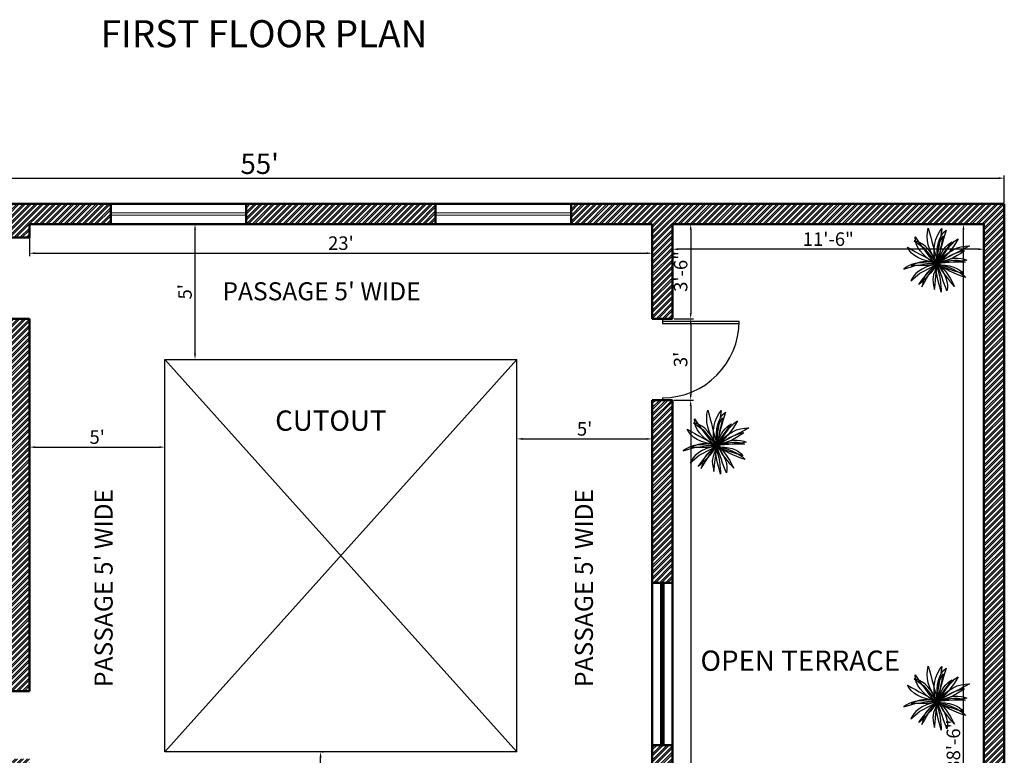
# Model space of a CAD drawing. Units: inches. Extents: x 3590 to 5167, y 65 to 1917.
# Tile 25 of 100: x 4644 to 5080, y 971 to 1297. Entities that reach past the tile are written whole.
import ezdxf

# ---------------------------------------------------------------- set-up
doc = ezdxf.new("R2010")
doc.units = ezdxf.units.IN
for name, color, linetype, lineweight in [('A-ANNO-DIMS', 2, 'Continuous', 18), ('A-ANNO-TEXT', 7, 'Continuous', 25), ('A-AREA-IDEN', 7, 'Continuous', 18), ('A-DOOR', 3, 'Continuous', 25), ('A-FLOR-OTLN', 7, 'Continuous', 25), ('A-GLAZ', 4, 'Continuous', 18), ('A-WALL', 7, 'Continuous', 50), ('A-WALL-PATT', 251, 'Continuous', 13), ('L-PLNT', 94, 'Continuous', 18)]:
    doc.layers.add(name, color=color, linetype=linetype, lineweight=lineweight)
doc.layers.add('DIENHOA', color=3, linetype='Continuous')
doc.styles.get("Standard").update_dxf_attribs({"font": 'arial.ttf'})
doc.dimstyles.new('ISO-25', dxfattribs={"dimtxt": 9, "dimasz": 2.5, "dimexe": 1.25, "dimexo": 0.625, "dimtad": 1, "dimdec": 1, "dimlunit": 3, "dimtxsty": 'Standard', "dimcen": 2.5, "dimadec": 0, "dimazin": 0, "dimtfac": 1, "dimtdec": 1, "dimtmove": 0, "dimatfit": 3, "dimfxl": 1, "dimarcsym": 0})

# ---------------------------------------------------------------- blocks, each defined once
blk = doc.blocks.new('*D105')
at = {"layer": 'A-ANNO-DIMS', "color": 0, "lineweight": -2, "transparency": 16777216}
for p, q in [((4420.27, 1215.97), (4420.27, 1227.96)), ((4422.77, 1226.71), (5077.77, 1226.71)), ((5080.27, 1215.97), (5080.27, 1227.96))]:
    blk.add_line(p, q, dxfattribs=at)
at = {"layer": 'A-ANNO-DIMS', "color": 0, "transparency": 16777216}
for points in [[(4422.77, 1227.13), (4422.77, 1226.29), (4420.27, 1226.71)], [(5077.77, 1227.13), (5077.77, 1226.29), (5080.27, 1226.71)]]:
    blk.add_solid(points, dxfattribs=at)
at = {"layer": 'Defpoints', "color": 0, "transparency": 16777216}
for p in [(5080.27, 1226.71), (4420.27, 1215.35), (5080.27, 1215.35)]:
    blk.add_point(p, dxfattribs=at)
at = {"layer": 'A-ANNO-DIMS', "color": 0, "transparency": 16777216, "insert": (4750.27, 1231.91), "char_height": 9, "attachment_point": 5}
blk.add_mtext("55'", dxfattribs=at)
blk = doc.blocks.new('Cay03_mb')
at = {"layer": 'DIENHOA'}
for p, q in [((79, 504), (119, 555)), ((119, 555), (166, 599)), ((166, 599), (142, 519)), ((-365, 390), (-414, 403)), ((-414, 403), (-240, 278)), ((-315, 371), (-365, 390)), ((-264, 343), (-315, 371)), ((10, 295), (25, 374)), ((25, 374), (49, 444)), ((49, 444), (79, 504)), ((97, 366), (76, 291)), ((119, 442), (97, 366)), ((142, 519), (119, 442)), ((-211, 305), (-264, 343)), ((-240, 278), (-88, 95)), ((-158, 252), (-211, 305)), ((-104, 184), (-158, 252)), ((-50, 98), (-104, 184)), ((0, 105), (2, 206)), ((2, 206), (10, 295)), ((56, 216), (37, 142)), ((76, 291), (56, 216)), ((147, 144), (219, 200)), ((219, 200), (291, 243)), ((364, 193), (290, 155)), ((291, 243), (363, 275)), ((363, 275), (437, 297)), ((438, 231), (364, 193)), ((437, 297), (511, 310)), ((512, 271), (438, 231)), ((511, 310), (586, 314)), ((586, 314), (512, 271)), ((-345, 5), (-400, -17)), ((-299, 20), (-345, 5)), ((-255, 27), (-299, 20)), ((-208, 28), (-255, 27)), ((-153, 22), (-208, 28)), ((-83, 10), (-153, 22)), ((-88, 95), (5, -8)), ((5, -8), (-83, 10)), ((5, -8), (-50, 98)), ((5, -8), (0, 105)), ((5, -8), (76, 75)), ((20, 68), (5, -8)), ((75, 36), (5, -8)), ((5, -8), (100, 18)), ((46, 1), (5, -8)), ((37, 142), (20, 68)), ((97, 7), (46, 1)), ((145, 77), (75, 36)), ((76, 75), (147, 144)), ((155, 12), (97, 7)), ((100, 18), (182, 37)), ((217, 117), (145, 77)), ((220, 15), (155, 12)), ((182, 37), (253, 49)), ((290, 155), (217, 117)), ((289, 17), (220, 15)), ((253, 49), (315, 54)), ((362, 19), (289, 17)), ((315, 54), (369, 53)), ((436, 19), (362, 19)), ((369, 53), (419, 47)), ((419, 47), (465, 35)), ((510, 19), (436, 19)), ((465, 35), (510, 19)), ((-400, -17), (-468, -48)), ((-468, -48), (-376, -38)), ((-376, -38), (-295, -28)), ((-295, -28), (-226, -19)), ((-226, -19), (-166, -11)), ((-216, -236), (-166, -174)), ((-166, -11), (-114, -6)), ((-166, -174), (-120, -122)), ((-120, -122), (-80, -80)), ((-75, -127), (-118, -181)), ((-114, -6), (-69, -3)), ((-80, -80), (-45, -46)), ((-33, -69), (-75, -127)), ((-69, -3), (-30, -3)), ((-45, -46), (-17, -22)), ((5, -8), (-33, -69)), ((-30, -3), (5, -8)), ((-17, -22), (5, -8)), ((5, -8), (57, -73)), ((26, -64), (5, -8)), ((5, -8), (113, -40)), ((53, -42), (5, -8)), ((47, -126), (26, -64)), ((69, -191), (47, -126)), ((107, -76), (53, -42)), ((57, -73), (100, -139)), ((100, -139), (136, -204)), ((166, -110), (107, -76)), ((113, -40), (207, -74)), ((229, -143), (166, -110)), ((207, -74), (290, -108)), ((296, -175), (229, -143)), ((290, -108), (359, -141)), ((367, -205), (296, -175)), ((359, -141), (417, -174)), ((417, -174), (463, -204)), ((-330, -387), (-271, -307)), ((-291, -355), (-330, -387)), ((-250, -318), (-291, -355)), ((-271, -307), (-216, -236)), ((-206, -276), (-250, -318)), ((-162, -231), (-206, -276)), ((-118, -181), (-162, -231)), ((91, -257), (69, -191)), ((113, -322), (91, -257)), ((135, -386), (113, -322)), ((136, -204), (163, -268)), ((163, -268), (181, -330)), ((181, -330), (190, -390)), ((442, -233), (367, -205)), ((519, -258), (442, -233)), ((463, -204), (496, -232)), ((496, -232), (519, -258)), ((158, -445), (135, -386)), ((180, -499), (158, -445)), ((190, -446), (180, -499)), ((190, -390), (190, -446))]:
    blk.add_line(p, q, dxfattribs=at)
for points in [[(24, -5), (-41, 82), (-92, 167), (-130, 249), (-156, 330), (-170, 408), (-175, 484), (-170, 559), (-157, 633)], [(-157, 633), (-132, 551), (-111, 470), (-90, 389), (-70, 309), (-49, 229), (-27, 150), (-3, 72), (24, -5)], [(-16, -27), (-38, 80), (-49, 178), (-49, 269), (-39, 353), (-19, 430), (9, 501), (45, 567), (88, 629)], [(88, 629), (75, 544), (61, 461), (46, 379), (31, 298), (16, 217), (3, 136), (-8, 55), (-16, -27)], [(-396, 474), (-348, 406), (-301, 339), (-254, 275), (-208, 212), (-162, 151), (-115, 91), (-66, 32), (-16, -27)], [(-16, -27), (-108, 39), (-187, 102), (-252, 163), (-305, 224), (-345, 285), (-374, 347), (-390, 409), (-396, 474)], [(273, 387), (228, 329), (182, 270), (138, 212), (97, 156), (60, 103), (28, 55), (2, 11), (-16, -27)], [(-16, -27), (21, 64), (57, 140), (91, 203), (125, 255), (160, 297), (195, 332), (233, 362), (273, 387)], [(24, -5), (20, 93), (20, 177), (25, 249), (34, 310), (47, 363), (65, 409), (87, 452), (113, 492)], [(113, 492), (96, 420), (79, 347), (64, 276), (50, 208), (38, 145), (30, 87), (25, 36), (24, -5)], [(384, 437), (342, 368), (298, 302), (253, 239), (206, 181), (159, 127), (113, 78), (68, 34), (24, -5)], [(24, -5), (80, 92), (134, 176), (186, 248), (234, 309), (279, 357), (319, 395), (355, 421), (384, 437)], [(-530, 290), (-458, 248), (-388, 208), (-319, 169), (-251, 131), (-183, 95), (-115, 60), (-46, 26), (24, -5)], [(24, -5), (-87, 15), (-185, 40), (-270, 68), (-344, 101), (-406, 140), (-457, 184), (-499, 233), (-530, 290)], [(497, 224), (429, 178), (362, 137), (294, 99), (227, 66), (162, 37), (100, 11), (40, -10), (-16, -27)], [(-16, -27), (75, 38), (160, 92), (237, 136), (307, 170), (368, 195), (420, 213), (463, 222), (497, 224)], [(-16, -27), (-134, -5), (-235, 5), (-322, 5), (-396, -5), (-459, -22), (-512, -46), (-558, -74), (-598, -105)], [(24, -5), (99, 30), (173, 57), (245, 77), (313, 88), (378, 92), (438, 87), (493, 74), (541, 52)], [(541, 52), (484, 43), (421, 35), (354, 28), (285, 21), (216, 14), (148, 8), (83, 2), (24, -5)], [(-598, -105), (-393, -44), (-155, -37), (-16, -27)], [(-472, -320), (-310, -179), (-98, -73), (24, -5)], [(24, -5), (-92, -35), (-188, -68), (-267, -105), (-330, -145), (-380, -187), (-418, -231), (-448, -275), (-472, -320)], [(-276, -424), (-227, -345), (-186, -276), (-150, -216), (-119, -164), (-91, -120), (-66, -82), (-41, -52), (-16, -27)], [(-16, -27), (-85, -86), (-137, -133), (-176, -173), (-204, -210), (-226, -249), (-243, -295), (-258, -352), (-276, -424)], [(24, -5), (-14, -88), (-41, -153), (-60, -205), (-70, -251), (-73, -295), (-69, -344), (-60, -402), (-45, -475)], [(-45, -475), (-34, -383), (-25, -303), (-18, -233), (-12, -173), (-6, -121), (2, -77), (11, -39), (24, -5)], [(76, -524), (49, -428), (27, -342), (9, -264), (-4, -196), (-12, -138), (-17, -90), (-18, -53), (-16, -27)], [(478, -192), (422, -176), (361, -157), (298, -135), (232, -113), (167, -89), (102, -67), (41, -45), (-16, -27)], [(-16, -27), (67, -27), (146, -33), (219, -45), (286, -63), (346, -87), (398, -117), (443, -152), (478, -192)], [(-16, -27), (8, -95), (29, -163), (44, -231), (56, -296), (65, -359), (71, -419), (74, -474), (76, -524)], [(316, -418), (251, -343), (195, -273), (147, -210), (106, -154), (74, -105), (50, -63), (33, -30), (24, -5)], [(24, -5), (75, -57), (122, -111), (164, -165), (203, -219), (237, -273), (267, -324), (294, -373), (316, -418)]]:
    blk.add_lwpolyline(points, dxfattribs=at)
blk = doc.blocks.new('D1')
for p, q in [((1, 0), (1, 34)), ((2, 0), (2, 33.99)), ((0, 0), (2, 0)), ((35, 0), (36, 0))]:
    blk.add_line(p, q)
at = {"ltscale": 0.5}
blk.add_arc((1, 0), 34, 0, 90, dxfattribs=at)
blk = doc.blocks.new('*D150')
at = {"layer": 'A-ANNO-DIMS', "color": 0, "lineweight": -2, "transparency": 16777216}
for p, q in [((5070.65, 1206.35), (5060.93, 1206.35)), ((5062.18, 746.85), (5062.18, 1203.85)), ((5070.65, 744.35), (5060.93, 744.35))]:
    blk.add_line(p, q, dxfattribs=at)
at = {"layer": 'A-ANNO-DIMS', "color": 0, "transparency": 16777216}
for points in [[(5061.77, 1203.85), (5062.6, 1203.85), (5062.18, 1206.35)], [(5061.77, 746.85), (5062.6, 746.85), (5062.18, 744.35)]]:
    blk.add_solid(points, dxfattribs=at)
at = {"layer": 'Defpoints', "color": 0, "transparency": 16777216}
for p in [(5062.18, 1206.35), (5071.27, 1206.35), (5071.27, 744.35)]:
    blk.add_point(p, dxfattribs=at)
at = {"layer": 'A-ANNO-DIMS', "color": 0, "transparency": 16777216, "insert": (5058.49, 975.35), "char_height": 6, "attachment_point": 5, "rotation": 90}
blk.add_mtext('38\'-6"', dxfattribs=at)
blk = doc.blocks.new('*D151')
at = {"layer": 'A-ANNO-DIMS', "color": 0, "lineweight": -2, "transparency": 16777216}
for p, q in [((4933.27, 1205.72), (4933.27, 1193.97)), ((5071.27, 1205.72), (5071.27, 1193.97)), ((5068.77, 1195.22), (4935.77, 1195.22))]:
    blk.add_line(p, q, dxfattribs=at)
at = {"layer": 'A-ANNO-DIMS', "color": 0, "transparency": 16777216}
for points in [[(4935.77, 1195.64), (4935.77, 1194.8), (4933.27, 1195.22)], [(5068.77, 1195.64), (5068.77, 1194.8), (5071.27, 1195.22)]]:
    blk.add_solid(points, dxfattribs=at)
at = {"layer": 'Defpoints', "color": 0, "transparency": 16777216}
for p in [(4933.27, 1206.35), (5071.27, 1206.35), (4933.27, 1195.22)]:
    blk.add_point(p, dxfattribs=at)
at = {"layer": 'A-ANNO-DIMS', "color": 0, "transparency": 16777216, "insert": (5002.27, 1198.91), "char_height": 6, "attachment_point": 5}
blk.add_mtext('11\'-6"', dxfattribs=at)
blk = doc.blocks.new('*D152')
at = {"layer": 'A-ANNO-DIMS', "color": 0, "lineweight": -2, "transparency": 16777216}
for p, q in [((4933.9, 1206.35), (4942.54, 1206.35)), ((4941.29, 1203.85), (4941.29, 1166.85)), ((4933.9, 1164.35), (4942.54, 1164.35))]:
    blk.add_line(p, q, dxfattribs=at)
at = {"layer": 'A-ANNO-DIMS', "color": 0, "transparency": 16777216}
for points in [[(4940.87, 1203.85), (4941.71, 1203.85), (4941.29, 1206.35)], [(4940.87, 1166.85), (4941.71, 1166.85), (4941.29, 1164.35)]]:
    blk.add_solid(points, dxfattribs=at)
at = {"layer": 'Defpoints', "color": 0, "transparency": 16777216}
for p in [(4933.27, 1206.35), (4933.27, 1164.35), (4941.29, 1164.35)]:
    blk.add_point(p, dxfattribs=at)
at = {"layer": 'A-ANNO-DIMS', "color": 0, "transparency": 16777216, "insert": (4937.6, 1185.35), "char_height": 6, "attachment_point": 5, "rotation": 90}
blk.add_mtext('3\'-6"', dxfattribs=at)
blk = doc.blocks.new('*D153')
at = {"layer": 'A-ANNO-DIMS', "color": 0, "lineweight": -2, "transparency": 16777216}
for p, q in [((4933.9, 1164.35), (4942.54, 1164.35)), ((4941.29, 1161.85), (4941.29, 1130.85)), ((4933.9, 1128.35), (4942.54, 1128.35))]:
    blk.add_line(p, q, dxfattribs=at)
at = {"layer": 'A-ANNO-DIMS', "color": 0, "transparency": 16777216}
for points in [[(4940.87, 1161.85), (4941.71, 1161.85), (4941.29, 1164.35)], [(4940.87, 1130.85), (4941.71, 1130.85), (4941.29, 1128.35)]]:
    blk.add_solid(points, dxfattribs=at)
at = {"layer": 'Defpoints', "color": 0, "transparency": 16777216}
for p in [(4933.27, 1164.35), (4933.27, 1128.35), (4941.29, 1128.35)]:
    blk.add_point(p, dxfattribs=at)
at = {"layer": 'A-ANNO-DIMS', "color": 0, "transparency": 16777216, "insert": (4937.6, 1146.35), "char_height": 6, "attachment_point": 5, "rotation": 90}
blk.add_mtext("3'", dxfattribs=at)
blk = doc.blocks.new('*D154')
at = {"layer": 'A-ANNO-DIMS', "color": 0, "lineweight": -2, "transparency": 16777216}
for p, q in [((4933.9, 1128.35), (4942.54, 1128.35)), ((4941.29, 1125.85), (4941.29, 746.85)), ((4933.9, 744.35), (4942.54, 744.35))]:
    blk.add_line(p, q, dxfattribs=at)
at = {"layer": 'A-ANNO-DIMS', "color": 0, "transparency": 16777216}
for points in [[(4940.87, 1125.85), (4941.71, 1125.85), (4941.29, 1128.35)], [(4940.87, 746.85), (4941.71, 746.85), (4941.29, 744.35)]]:
    blk.add_solid(points, dxfattribs=at)
at = {"layer": 'Defpoints', "color": 0, "transparency": 16777216}
for p in [(4933.27, 1128.35), (4933.27, 744.35), (4941.29, 744.35)]:
    blk.add_point(p, dxfattribs=at)
at = {"layer": 'A-ANNO-DIMS', "color": 0, "transparency": 16777216, "insert": (4937.6, 936.35), "char_height": 6, "attachment_point": 5, "rotation": 90}
blk.add_mtext("32'", dxfattribs=at)
blk = doc.blocks.new('*D155')
at = {"layer": 'A-ANNO-DIMS', "color": 0, "lineweight": -2, "transparency": 16777216}
for p, q in [((4648.27, 1205.72), (4648.27, 1192.19)), ((4924.27, 1205.72), (4924.27, 1192.19)), ((4650.77, 1193.44), (4921.77, 1193.44))]:
    blk.add_line(p, q, dxfattribs=at)
at = {"layer": 'A-ANNO-DIMS', "color": 0, "transparency": 16777216}
for points in [[(4650.77, 1193.86), (4650.77, 1193.02), (4648.27, 1193.44)], [(4921.77, 1193.86), (4921.77, 1193.02), (4924.27, 1193.44)]]:
    blk.add_solid(points, dxfattribs=at)
at = {"layer": 'Defpoints', "color": 0, "transparency": 16777216}
for p in [(4648.27, 1206.35), (4924.27, 1206.35), (4924.27, 1193.44)]:
    blk.add_point(p, dxfattribs=at)
at = {"layer": 'A-ANNO-DIMS', "color": 0, "transparency": 16777216, "insert": (4786.27, 1197.13), "char_height": 6, "attachment_point": 5}
blk.add_mtext("23'", dxfattribs=at)
blk = doc.blocks.new('*D156')
at = {"layer": 'A-ANNO-DIMS', "color": 0, "lineweight": -2, "transparency": 16777216}
for p, q in [((4708.27, 1108.1), (4708.27, 1108.73)), ((4648.27, 1106.85), (4648.27, 1106.23)), ((4650.77, 1107.48), (4705.77, 1107.48))]:
    blk.add_line(p, q, dxfattribs=at)
at = {"layer": 'A-ANNO-DIMS', "color": 0, "transparency": 16777216}
for points in [[(4650.77, 1107.89), (4650.77, 1107.06), (4648.27, 1107.48)], [(4705.77, 1107.89), (4705.77, 1107.06), (4708.27, 1107.48)]]:
    blk.add_solid(points, dxfattribs=at)
at = {"layer": 'Defpoints', "color": 0, "transparency": 16777216}
for p in [(4648.27, 1107.48), (4708.27, 1107.48), (4708.27, 1107.48)]:
    blk.add_point(p, dxfattribs=at)
at = {"layer": 'A-ANNO-DIMS', "color": 0, "transparency": 16777216, "insert": (4678.27, 1111.15), "char_height": 6, "attachment_point": 5}
blk.add_mtext("5'", dxfattribs=at)
blk = doc.blocks.new('*D157')
at = {"layer": 'A-ANNO-DIMS', "color": 0, "lineweight": -2, "transparency": 16777216}
for p, q in [((4722.25, 1206.35), (4722.88, 1206.35)), ((4721.63, 1148.85), (4721.63, 1203.85)), ((4722.25, 1146.35), (4722.88, 1146.35))]:
    blk.add_line(p, q, dxfattribs=at)
at = {"layer": 'A-ANNO-DIMS', "color": 0, "transparency": 16777216}
for points in [[(4721.21, 1203.85), (4722.04, 1203.85), (4721.63, 1206.35)], [(4721.21, 1148.85), (4722.04, 1148.85), (4721.63, 1146.35)]]:
    blk.add_solid(points, dxfattribs=at)
at = {"layer": 'Defpoints', "color": 0, "transparency": 16777216}
for p in [(4721.63, 1206.35), (4721.63, 1206.35), (4721.63, 1146.35)]:
    blk.add_point(p, dxfattribs=at)
at = {"layer": 'A-ANNO-DIMS', "color": 0, "transparency": 16777216, "insert": (4717.95, 1176.35), "char_height": 6, "attachment_point": 5, "rotation": 90}
blk.add_mtext("5'", dxfattribs=at)
blk = doc.blocks.new('*D158')
at = {"layer": 'A-ANNO-DIMS', "color": 0, "lineweight": -2, "transparency": 16777216}
for p, q in [((4777.27, 914.85), (4777.27, 969.85)), ((4777.9, 972.35), (4778.52, 972.35)), ((4777.9, 912.35), (4778.52, 912.35))]:
    blk.add_line(p, q, dxfattribs=at)
at = {"layer": 'A-ANNO-DIMS', "color": 0, "transparency": 16777216}
for points in [[(4776.86, 969.85), (4777.69, 969.85), (4777.27, 972.35)], [(4776.86, 914.85), (4777.69, 914.85), (4777.27, 912.35)]]:
    blk.add_solid(points, dxfattribs=at)
at = {"layer": 'Defpoints', "color": 0, "transparency": 16777216}
for p in [(4777.27, 972.35), (4777.27, 972.35), (4777.27, 912.35)]:
    blk.add_point(p, dxfattribs=at)
at = {"layer": 'A-ANNO-DIMS', "color": 0, "transparency": 16777216, "insert": (4773.6, 942.35), "char_height": 6, "attachment_point": 5, "rotation": 90}
blk.add_mtext("5'", dxfattribs=at)
blk = doc.blocks.new('*D159')
at = {"layer": 'A-ANNO-DIMS', "color": 0, "lineweight": -2, "transparency": 16777216}
for p, q in [((4864.27, 1111.74), (4864.27, 1112.37)), ((4866.77, 1111.12), (4921.77, 1111.12)), ((4924.27, 1111.74), (4924.27, 1112.37))]:
    blk.add_line(p, q, dxfattribs=at)
at = {"layer": 'A-ANNO-DIMS', "color": 0, "transparency": 16777216}
for points in [[(4866.77, 1111.53), (4866.77, 1110.7), (4864.27, 1111.12)], [(4921.77, 1111.53), (4921.77, 1110.7), (4924.27, 1111.12)]]:
    blk.add_solid(points, dxfattribs=at)
at = {"layer": 'Defpoints', "color": 0, "transparency": 16777216}
for p in [(4864.27, 1111.12), (4924.27, 1111.12), (4924.27, 1111.12)]:
    blk.add_point(p, dxfattribs=at)
at = {"layer": 'A-ANNO-DIMS', "color": 0, "transparency": 16777216, "insert": (4894.27, 1114.79), "char_height": 6, "attachment_point": 5}
blk.add_mtext("5'", dxfattribs=at)

msp = doc.modelspace()

# ---------------------------------------------------------------- hatches: boundary and pattern name
at = {"layer": 'A-WALL-PATT', "transparency": 33554687}
h = msp.add_hatch(dxfattribs=at)
h.set_pattern_fill('ANSI32', color=256, scale=0.2)
h.set_pattern_definition([(45, (0, -590.6538), (-1.3470384, 1.3470384), []), (45, (0.898, -590.6538), (-1.3470384, 1.3470384), [])])
h.paths.add_polyline_path([(4684.27, 1215.35), (4591.27, 1215.35), (4591.27, 1206.35), (4639.27, 1206.35), (4639.27, 1200.35), (4648.27, 1200.35), (4648.27, 1206.35), (4684.27, 1206.35)])
h.paths.add_polyline_path([(4543.27, 1215.35), (4420.27, 1215.35), (4420.27, 1194.35), (4429.27, 1194.35), (4429.27, 1206.35), (4445.92, 1206.35), (4543.27, 1206.35)])
h.paths.add_polyline_path([(4828.27, 1215.35), (4744.27, 1215.35), (4744.27, 1206.35), (4828.27, 1206.35)])
h.paths.add_polyline_path([(4648.27, 1164.35), (4639.27, 1164.35), (4639.27, 1065.35), (4546.27, 1065.35), (4546.27, 1059.35), (4549.27, 1059.35), (4549.27, 963.35), (4429.27, 963.35), (4429.27, 993.35), (4420.27, 993.35), (4420.27, 948.35), (4429.27, 948.35), (4429.27, 954.35), (4639.27, 954.35), (4639.27, 948.35), (4648.27, 948.35), (4648.27, 969.35), (4639.27, 969.35), (4639.27, 963.35), (4555.27, 963.35), (4555.27, 1059.35), (4639.27, 1059.35), (4639.27, 999.35), (4648.27, 999.35)])
h.paths.add_polyline_path([(4516.27, 1065.35), (4429.27, 1065.35), (4429.27, 1146.35), (4420.27, 1146.35), (4420.27, 1029.35), (4429.27, 1029.35), (4429.27, 1059.35), (4516.27, 1059.35)], flags=17)
h.paths.add_polyline_path([(5080.27, 1215.35), (4888.27, 1215.35), (4888.27, 1206.35), (4924.27, 1206.35), (4924.27, 1164.35), (4933.27, 1164.35), (4933.27, 1206.35), (5071.27, 1206.35), (5071.27, 744.35), (4933.27, 744.35), (4933.27, 975.35), (4924.27, 975.35), (4924.27, 744.35), (4898.77, 744.35), (4898.77, 735.35), (5080.27, 735.35)])
h.paths.add_polyline_path([(4933.27, 1128.35), (4924.27, 1128.35), (4924.27, 1047.35), (4933.27, 1047.35)], flags=17)
h.paths.add_polyline_path([(4802.77, 744.35), (4777.27, 744.35), (4777.27, 912.35), (4756.27, 912.35), (4756.27, 903.35), (4768.27, 903.35), (4768.27, 840.35), (4696.27, 840.35), (4696.27, 903.35), (4708.27, 903.35), (4708.27, 912.35), (4639.27, 912.35), (4639.27, 903.35), (4687.27, 903.35), (4687.27, 840.35), (4681.27, 840.35), (4681.27, 831.35), (4768.27, 831.35), (4768.27, 744.35), (4726.27, 744.35), (4726.27, 735.35), (4802.77, 735.35)])
h.paths.add_polyline_path([(4690.27, 744.35), (4648.27, 744.35), (4648.27, 762.21), (4648.27, 831.35), (4651.27, 831.35), (4651.27, 840.35), (4639.27, 840.35), (4639.27, 744.35), (4633.27, 744.35), (4633.27, 735.35), (4690.27, 735.35)])
h.paths.add_polyline_path([(4585.27, 744.35), (4584.72, 744.35), (4429.27, 744.35), (4429.27, 900.35), (4420.27, 900.35), (4420.27, 735.35), (4585.27, 735.35)])

# ---------------------------------------------------------------- linework, layer by layer
at = {"layer": 'A-FLOR-OTLN'}
for p, q in [((4708.27, 1146.35), (4864.27, 1146.35)), ((4708.27, 972.35), (4708.27, 1146.35)), ((4864.27, 972.35), (4864.27, 1146.35)), ((4864.27, 972.35), (4708.27, 972.35))]:
    msp.add_line(p, q, dxfattribs=at)
at = {"layer": 'A-FLOR-OTLN', "ltscale": 0.5}
for p, q in [((4708.27, 1146.35), (4864.27, 972.35)), ((4708.27, 972.35), (4864.27, 1146.35))]:
    msp.add_line(p, q, dxfattribs=at)
at = {"layer": 'A-GLAZ'}
for p, q in [((4744.27, 1211.35), (4684.27, 1211.35)), ((4744.27, 1210.35), (4684.27, 1210.35)), ((4888.27, 1211.35), (4828.27, 1211.35)), ((4888.27, 1210.35), (4828.27, 1210.35))]:
    msp.add_line(p, q, dxfattribs=at)
at = {"layer": 'A-WALL'}
for p, q in [((4684.27, 1206.35), (4684.27, 1215.35)), ((4744.27, 1206.35), (4744.27, 1215.35)), ((4828.27, 1206.35), (4828.27, 1215.35)), ((4888.27, 1206.35), (4888.27, 1215.35)), ((4648.27, 1206.35), (4924.27, 1206.35)), ((4648.27, 1200.35), (4648.27, 1206.35)), ((4924.27, 1164.35), (4924.27, 1206.35)), ((4933.27, 1206.35), (5071.27, 1206.35)), ((4933.27, 1164.35), (4933.27, 1206.35)), ((5071.27, 744.35), (5071.27, 1206.35)), ((4639.27, 1200.35), (4648.27, 1200.35)), ((4639.27, 1164.35), (4648.27, 1164.35)), ((4648.27, 999.35), (4648.27, 1164.35)), ((4924.27, 1164.35), (4933.27, 1164.35)), ((4924.27, 744.35), (4924.27, 1128.35)), ((4924.27, 1128.35), (4933.27, 1128.35)), ((4933.27, 744.35), (4933.27, 1128.35)), ((4924.27, 1047.35), (4933.27, 1047.35)), ((4928.27, 975.35), (4928.27, 1047.35)), ((4929.27, 975.35), (4929.27, 1047.35)), ((4648.27, 999.35), (4639.27, 999.35)), ((4924.27, 975.35), (4933.27, 975.35))]:
    msp.add_line(p, q, dxfattribs=at)
msp.add_lwpolyline([(5080.27, 1215.35), (5080.27, 735.35), (4420.27, 735.35), (4420.27, 1215.35)], close=True, dxfattribs=at)

# ---------------------------------------------------------------- block references
at = {"layer": 'A-DOOR', "rotation": 270}
msp.add_blockref('D1', (4928.77, 1164.35), dxfattribs=at)
at = {"layer": 'L-PLNT', "xscale": 0.0245452446402784, "yscale": 0.0245452446402784, "zscale": 0.0245452446402784}
for p in [(5050.43, 1189.02), (4952.67, 1108.34), (5050.43, 994.85)]:
    msp.add_blockref('Cay03_mb', p, dxfattribs=at)

# ---------------------------------------------------------------- texts
at = {"layer": 'A-ANNO-TEXT', "insert": (4679.79, 1296.76), "char_height": 12, "attachment_point": 1}
msp.add_mtext_dynamic_manual_height_columns('{\\fTimes New Roman|b0|i0|c0|p18;FIRST FLOOR PLAN}', width=197.6934, gutter_width=12.5, heights=[0], dxfattribs=at)
at = {"layer": 'A-AREA-IDEN', "attachment_point": 1}
for s, width, insert, char_height in [("{\\fTimes New Roman|b0|i0|c0|p18;PASSAGE 5' WIDE}", 131.4857, (4733.77, 1180.57), 8), ('{\\fTimes New Roman|b0|i0|c0|p18;CUTOUT}', 98.8219, (4757.14, 1123.72), 9), ('{\\fTimes New Roman|b0|i0|c0|p18;OPEN TERRACE}', 98.8219, (4945.63, 1017.3), 9)]:
    msp.add_mtext_dynamic_manual_height_columns(s, width=width, gutter_width=12.5, heights=[0], dxfattribs=dict(at, insert=insert, char_height=char_height))
at = {"layer": 'A-AREA-IDEN', "char_height": 8, "attachment_point": 1, "rotation": 90}
for insert in [(4677.11, 1001.12), (4889.96, 1001.12)]:
    msp.add_mtext_dynamic_manual_height_columns("{\\fTimes New Roman|b0|i0|c0|p18;PASSAGE 5' WIDE}", width=131.4857, gutter_width=12.5, heights=[0], dxfattribs=dict(at, insert=insert))

# ---------------------------------------------------------------- dimensions: what is measured, and where the dimension line sits
at = {"layer": 'A-ANNO-DIMS'}
for base, p1, p2, override, picture, middle in [((5080.27, 1226.71), (4420.27, 1215.35), (5080.27, 1215.35), {"dimclrd": 0, "dimclre": 0, "dimclrt": 0}, '*D105', (4750.27, 1231.91)), ((4924.27, 1193.44), (4648.27, 1206.35), (4924.27, 1206.35), {"dimtxt": 6, "dimclrd": 0, "dimclre": 0, "dimclrt": 0}, '*D155', (4786.27, 1197.13)), ((4933.27, 1195.22), (5071.27, 1206.35), (4933.27, 1206.35), {"dimtxt": 6, "dimclrd": 0, "dimclre": 0, "dimclrt": 0}, '*D151', (5002.27, 1198.91)), ((4924.27, 1111.12), (4864.27, 1111.12), (4924.27, 1111.12), {"dimtxt": 6, "dimclrd": 0, "dimclre": 0, "dimclrt": 0}, '*D159', (4894.27, 1114.79)), ((4708.27, 1107.48), (4648.27, 1107.48), (4708.27, 1107.48), {"dimtxt": 6, "dimclrd": 0, "dimclre": 0, "dimclrt": 0}, '*D156', (4678.27, 1111.15))]:
    dim = msp.add_linear_dim(base=base, p1=p1, p2=p2, dimstyle='ISO-25', override=override, dxfattribs=at)
    dim.commit()
    dim.dimension.update_dxf_attribs({"geometry": picture, "text_midpoint": middle})
for base, p1, p2, override, picture, middle in [((4721.63, 1206.35), (4721.63, 1146.35), (4721.63, 1206.35), {"dimtxt": 6, "dimclrd": 0, "dimclre": 0, "dimclrt": 0}, '*D157', (4717.95, 1176.35)), ((4941.29, 1164.35), (4933.27, 1206.35), (4933.27, 1164.35), {"dimtxt": 6, "dimclrd": 0, "dimclre": 0, "dimclrt": 0}, '*D152', (4937.6, 1185.35)), ((5062.18, 1206.35), (5071.27, 744.35), (5071.27, 1206.35), {"dimtxt": 6, "dimclrd": 0, "dimclre": 0, "dimclrt": 0}, '*D150', (5058.49, 975.35)), ((4941.29, 1128.35), (4933.27, 1164.35), (4933.27, 1128.35), {"dimtxt": 6, "dimclrd": 0, "dimclre": 0, "dimclrt": 0, "dimtmove": 1}, '*D153', (4937.6, 1146.35)), ((4941.29, 744.35), (4933.27, 1128.35), (4933.27, 744.35), {"dimtxt": 6, "dimclrd": 0, "dimclre": 0, "dimclrt": 0, "dimtmove": 1}, '*D154', (4937.6, 936.35)), ((4777.27, 972.35), (4777.27, 912.35), (4777.27, 972.35), {"dimtxt": 6, "dimclrd": 0, "dimclre": 0, "dimclrt": 0}, '*D158', (4773.6, 942.35))]:
    dim = msp.add_linear_dim(base=base, p1=p1, p2=p2, angle=90, dimstyle='ISO-25', override=override, dxfattribs=at)
    dim.commit()
    dim.dimension.update_dxf_attribs({"geometry": picture, "text_midpoint": middle})

doc.saveas('drawing.dxf')
